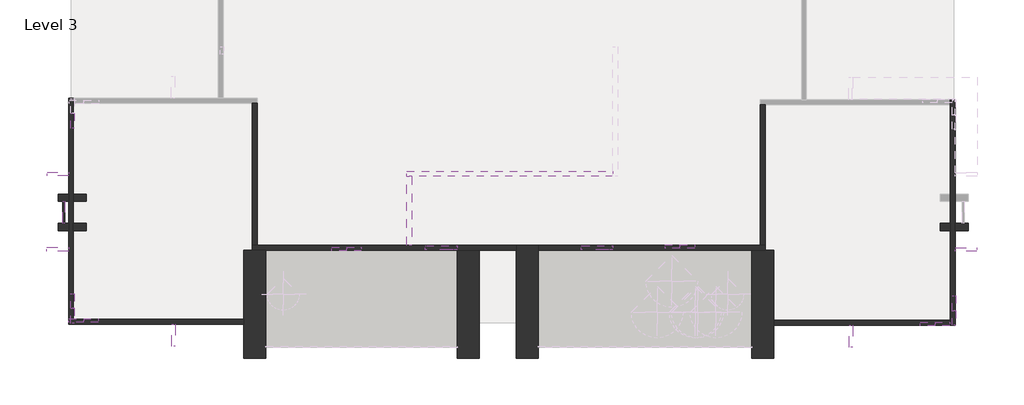
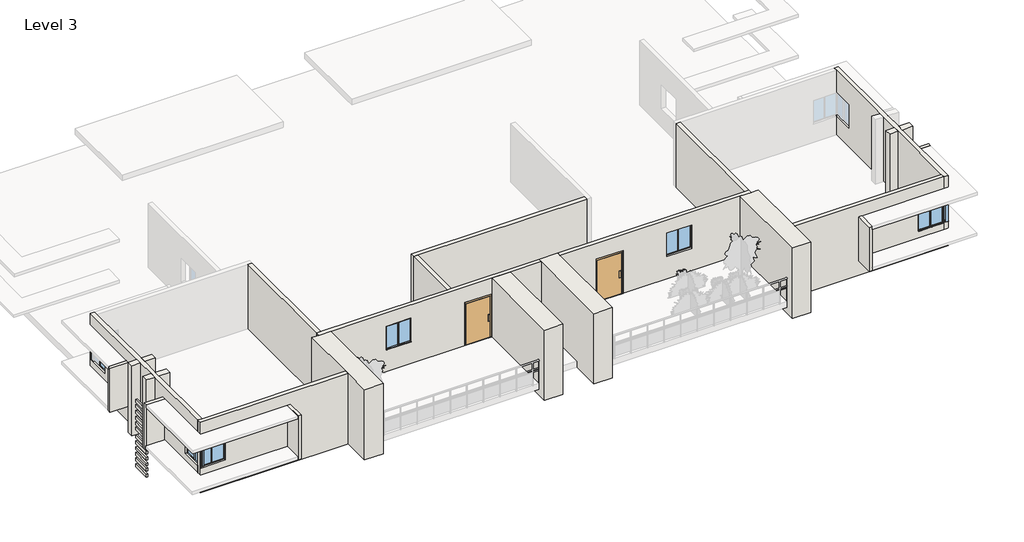
# One storey, part 1 of 4: 49 walls, 13 windows, 2 doors.
"""IFC4 building model written with IfcOpenShell, lengths in millimetres."""

from ifc_helpers import new_model, si_unit, frame, origin, place, context, project, spatial, polyline, outline, extrude, faceted_brep, transform, mapped, element, save
from components import door_15d3c954, window_20ff4747

model = new_model("IFC4")

# Units and contexts
model_context = context("Model", 3, world=origin())
ifc_project = project(units=[si_unit("LENGTHUNIT", "METRE", prefix="MILLI")], contexts=[model_context])

# Site, building, storey
site = spatial("IfcSite", under=ifc_project)
building = spatial("IfcBuilding", under=site)
storey = spatial("IfcBuildingStorey", under=building, Name="Level 3", Elevation=6096.0)

# Doors
placement = place(None, origin())
door_shape = door_15d3c954(model_context)
element("IfcDoor", 1, ObjectType="Door-Passage-Single-Flush-Dbl_Acting : 48\" x 96\"", at=placement, inside=storey, context=model_context, shape_type="MappedRepresentation", body=[
    mapped(door_shape, transform((7011.0520665, -5255.880811, 7315.2), x_axis=(-1.0, 0.0, 0.0), y_axis=(0.0, -1.0, 0.0), z_axis=(0.0, 0.0, 1.0))),
])
element("IfcDoor", 2, ObjectType="Door-Passage-Single-Flush-Dbl_Acting : 48\" x 96\"", at=placement, inside=storey, context=model_context, shape_type="MappedRepresentation", body=[
    mapped(door_shape, transform((559.4520665, -5255.1961695, 7315.2), x_axis=(-1.0, 0.0, 0.0), y_axis=(0.0, -1.0, 0.0), z_axis=(0.0, 0.0, 1.0))),
])

# Walls
element("IfcWall", 3, ObjectType="Generic - 1'", at=placement, inside=storey, context=model_context, shape_type="SweptSolid", body=[
    extrude(outline(polyline([(-14151.7972154, -3343.5294056), (-14680.5479335, -3343.5294056), (-14680.5479335, -3038.7294056), (-14151.7972154, -3038.7294056), (-14151.7972154, -3343.5294056)])), frame((0.0, 0.0, 6705.6), z_axis=(0.0, 0.0, 1.0), x_axis=(1.0, 0.0, 0.0)), (0.0, 0.0, 1.0), 3657.6),
])
element("IfcWall", 4, ObjectType="Generic - 1'", at=placement, inside=storey, context=model_context, shape_type="SweptSolid", body=[
    extrude(outline(polyline([(-15302.1394029, -3038.7294056), (-14883.7479335, -3038.7294056), (-14883.7479335, -3343.5294056), (-15302.1394029, -3343.5294056), (-15302.1394029, -3038.7294056)])), frame((0.0, 0.0, 6705.6), z_axis=(0.0, 0.0, 1.0), x_axis=(1.0, 0.0, 0.0)), (0.0, 0.0, 1.0), 3657.6),
])
element("IfcWall", 5, ObjectType="Generic - 1'", at=placement, inside=storey, context=model_context, shape_type="SweptSolid", body=[
    extrude(outline(polyline([(-14151.7972154, -4562.7294056), (-14680.5479335, -4562.7294056), (-14680.5479335, -4257.9294056), (-14151.7972154, -4257.9294056), (-14151.7972154, -4562.7294056)])), frame((0.0, 0.0, 6705.6), z_axis=(0.0, 0.0, 1.0), x_axis=(1.0, 0.0, 0.0)), (0.0, 0.0, 1.0), 3657.6),
])
element("IfcWall", 6, ObjectType="Generic - 1'", at=placement, inside=storey, context=model_context, shape_type="SweptSolid", body=[
    extrude(outline(polyline([(-15302.1394029, -4257.9294056), (-14883.7479335, -4257.9294056), (-14883.7479335, -4562.7294056), (-15302.1394029, -4562.7294056), (-15302.1394029, -4257.9294056)])), frame((0.0, 0.0, 6705.6), z_axis=(0.0, 0.0, 1.0), x_axis=(1.0, 0.0, 0.0)), (0.0, 0.0, 1.0), 3657.6),
])
element("IfcWall", 7, ObjectType="Generic - 1'", at=placement, inside=storey, context=model_context, shape_type="SweptSolid", body=[
    extrude(outline(polyline([(22386.1027846, -4562.7294056), (21857.3520665, -4562.7294056), (21857.3520665, -4257.9294056), (22386.1027846, -4257.9294056), (22386.1027846, -4562.7294056)])), frame((0.0, 0.0, 6705.6), z_axis=(0.0, 0.0, 1.0), x_axis=(1.0, 0.0, 0.0)), (0.0, 0.0, 1.0), 3657.6),
])
element("IfcWall", 8, ObjectType="Generic - 1'", at=placement, inside=storey, context=model_context, shape_type="SweptSolid", body=[
    extrude(outline(polyline([(21235.7605971, -4257.9294056), (21654.1520665, -4257.9294056), (21654.1520665, -4562.7294056), (21235.7605971, -4562.7294056), (21235.7605971, -4257.9294056)])), frame((0.0, 0.0, 6705.6), z_axis=(0.0, 0.0, 1.0), x_axis=(1.0, 0.0, 0.0)), (0.0, 0.0, 1.0), 3657.6),
])
element("IfcWall", 9, ObjectType="Generic - 3'", at=placement, inside=storey, context=model_context, shape_type="Brep", body=[
    faceted_brep([(2134.2520665, -9833.5461695, 6705.6), (2134.2520665, -5363.1461695, 6705.6), (2134.2520665, -5363.1461695, 10363.2), (2134.2520665, -9833.5461695, 10363.2), (1219.8520665, -9833.5461695, 6705.6), (1219.8520665, -9833.5461695, 10363.2), (1219.8520665, -5363.1461695, 10363.2), (1219.8520665, -5363.1461695, 9550.4), (1219.8520665, -5363.1461695, 7315.2), (1219.8520665, -5363.1461695, 6705.6)], [[[0, 1, 2, 3]], [[4, 5, 6, 7, 8, 9]], [[1, 0, 4, 9]], [[3, 2, 6, 5]], [[0, 3, 5, 4]], [[2, 1, 9, 8, 7, 6]]]),
])
element("IfcWall", 10, ObjectType="Generic - 3'", at=placement, inside=storey, context=model_context, shape_type="Brep", body=[
    faceted_brep([(4572.6520665, -9833.5461695, 6705.6), (4572.6520665, -5363.830811, 6705.6), (4572.6520665, -5160.630811, 6705.6), (4572.6520665, -5160.630811, 10363.2), (4572.6520665, -5363.830811, 10363.2), (4572.6520665, -9833.5461695, 10363.2), (3658.2520665, -9833.5461695, 6705.6), (3658.2520665, -9833.5461695, 10363.2), (3658.2520665, -5363.1461695, 10363.2), (3658.2520665, -5160.630811, 10363.2), (3658.2520665, -5160.630811, 6705.6), (3658.2520665, -5363.1461695, 6705.6)], [[[0, 1, 2, 3, 4, 5]], [[6, 7, 8, 9, 10, 11]], [[2, 1, 0, 6, 11, 10]], [[5, 4, 3, 9, 8, 7]], [[0, 5, 7, 6]], [[3, 2, 10, 9]]]),
])
element("IfcWall", 11, ObjectType="Generic - 3'", at=placement, inside=storey, context=model_context, shape_type="Brep", body=[
    faceted_brep([(-7619.3479335, -5363.1461695, 6705.6), (-7619.3479335, -8237.0604699, 6705.6), (-7619.3479335, -8440.2604699, 6705.6), (-7619.3479335, -9833.5461695, 6705.6), (-7619.3479335, -9833.5461695, 10363.2), (-7619.3479335, -8440.2604699, 10363.2), (-7619.3479335, -8237.0604699, 10363.2), (-7619.3479335, -5363.1461695, 10363.2), (-6704.9479335, -5363.1461695, 6705.6), (-6704.9479335, -5363.1461695, 10363.2), (-6704.9479335, -9833.5461695, 10363.2), (-6704.9479335, -9833.5461695, 6705.6), (-7263.7479335, -5363.1461695, 6705.6), (-7263.7479335, -5363.1461695, 10363.2)], [[[0, 1, 2, 3, 4, 5, 6, 7]], [[8, 9, 10, 11]], [[3, 2, 1, 0, 12, 8, 11]], [[4, 3, 11, 10]], [[7, 6, 5, 4, 10, 9, 13]], [[0, 7, 13, 9, 8, 12]]]),
])
element("IfcWall", 12, ObjectType="Generic - 3'", at=placement, inside=storey, context=model_context, shape_type="Brep", body=[
    faceted_brep([(13411.8520665, -5363.830811, 6705.6), (13411.8520665, -9834.230811, 6705.6), (13411.8520665, -9834.230811, 10363.2), (13411.8520665, -5363.830811, 10363.2), (14326.2520665, -5363.830811, 6705.6), (14326.2520665, -5363.830811, 10363.2), (14326.2520665, -8263.1451114, 10363.2), (14326.2520665, -8466.3451114, 10363.2), (14326.2520665, -9834.230811, 10363.2), (14326.2520665, -9834.230811, 6705.6), (14326.2520665, -8466.3451114, 6705.6), (14326.2520665, -8263.1451114, 6705.6), (13970.6520665, -5363.830811, 6705.6), (13970.6520665, -5363.830811, 10363.2)], [[[0, 1, 2, 3]], [[4, 5, 6, 7, 8, 9, 10, 11]], [[1, 0, 12, 4, 11, 10, 9]], [[2, 1, 9, 8]], [[3, 2, 8, 7, 6, 5, 13]], [[0, 3, 13, 5, 4, 12]]]),
])
element("IfcWall", 13, ObjectType="Generic - 5\"", at=placement, inside=storey, context=model_context, shape_type="SweptSolid", body=[
    extrude(outline(polyline([(-15124.6936682, -4257.9294056), (-15124.6936682, -3343.5294056), (-15048.4936682, -3343.5294056), (-15048.4936682, -4257.9294056), (-15124.6936682, -4257.9294056)])), frame((0.0, 0.0, 5054.6), z_axis=(0.0, 0.0, 1.0), x_axis=(1.0, 0.0, 0.0)), (0.0, 0.0, 1.0), 152.8735856),
])
element("IfcWall", 14, ObjectType="Generic - 5\"", at=placement, inside=storey, context=model_context, shape_type="SweptSolid", body=[
    extrude(outline(polyline([(-15124.6936682, -4257.9294056), (-15124.6936682, -3343.5294056), (-15048.4936682, -3343.5294056), (-15048.4936682, -4257.9294056), (-15124.6936682, -4257.9294056)])), frame((0.0, 0.0, 5359.4), z_axis=(0.0, 0.0, 1.0), x_axis=(1.0, 0.0, 0.0)), (0.0, 0.0, 1.0), 152.8735856),
])
element("IfcWall", 15, ObjectType="Generic - 5\"", at=placement, inside=storey, context=model_context, shape_type="SweptSolid", body=[
    extrude(outline(polyline([(-15124.6936682, -4257.9294056), (-15124.6936682, -3343.5294056), (-15048.4936682, -3343.5294056), (-15048.4936682, -4257.9294056), (-15124.6936682, -4257.9294056)])), frame((0.0, 0.0, 5638.8), z_axis=(0.0, 0.0, 1.0), x_axis=(1.0, 0.0, 0.0)), (0.0, 0.0, 1.0), 152.8735856),
])
element("IfcWall", 16, ObjectType="Generic - 5\"", at=placement, inside=storey, context=model_context, shape_type="SweptSolid", body=[
    extrude(outline(polyline([(-15124.6936682, -4257.9294056), (-15124.6936682, -3343.5294056), (-15048.4936682, -3343.5294056), (-15048.4936682, -4257.9294056), (-15124.6936682, -4257.9294056)])), frame((0.0, 0.0, 5943.6), z_axis=(0.0, 0.0, 1.0), x_axis=(1.0, 0.0, 0.0)), (0.0, 0.0, 1.0), 152.8735856),
])
element("IfcWall", 17, ObjectType="Generic - 5\"", at=placement, inside=storey, context=model_context, shape_type="SweptSolid", body=[
    extrude(outline(polyline([(-15124.6936682, -4257.9294056), (-15124.6936682, -3343.5294056), (-15048.4936682, -3343.5294056), (-15048.4936682, -4257.9294056), (-15124.6936682, -4257.9294056)])), frame((0.0, 0.0, 6248.4), z_axis=(0.0, 0.0, 1.0), x_axis=(1.0, 0.0, 0.0)), (0.0, 0.0, 1.0), 152.8735856),
])
element("IfcWall", 18, ObjectType="Generic - 5\"", at=placement, inside=storey, context=model_context, shape_type="SweptSolid", body=[
    extrude(outline(polyline([(-15124.6936682, -4257.9294056), (-15124.6936682, -3343.5294056), (-15048.4936682, -3343.5294056), (-15048.4936682, -4257.9294056), (-15124.6936682, -4257.9294056)])), frame((0.0, 0.0, 6553.2), z_axis=(0.0, 0.0, 1.0), x_axis=(1.0, 0.0, 0.0)), (0.0, 0.0, 1.0), 152.8735856),
])
element("IfcWall", 19, ObjectType="Generic - 5\"", at=placement, inside=storey, context=model_context, shape_type="SweptSolid", body=[
    extrude(outline(polyline([(-15124.6936682, -4257.9294056), (-15124.6936682, -3343.5294056), (-15048.4936682, -3343.5294056), (-15048.4936682, -4257.9294056), (-15124.6936682, -4257.9294056)])), frame((0.0, 0.0, 5054.6), z_axis=(0.0, 0.0, 1.0), x_axis=(1.0, 0.0, 0.0)), (0.0, 0.0, 1.0), 152.8735856),
])
element("IfcWall", 20, ObjectType="Generic - 5\"", at=placement, inside=storey, context=model_context, shape_type="SweptSolid", body=[
    extrude(outline(polyline([(-15124.6936682, -4257.9294056), (-15124.6936682, -3343.5294056), (-15048.4936682, -3343.5294056), (-15048.4936682, -4257.9294056), (-15124.6936682, -4257.9294056)])), frame((0.0, 0.0, 5359.4), z_axis=(0.0, 0.0, 1.0), x_axis=(1.0, 0.0, 0.0)), (0.0, 0.0, 1.0), 152.8735856),
])
element("IfcWall", 21, ObjectType="Generic - 5\"", at=placement, inside=storey, context=model_context, shape_type="SweptSolid", body=[
    extrude(outline(polyline([(-15124.6936682, -4257.9294056), (-15124.6936682, -3343.5294056), (-15048.4936682, -3343.5294056), (-15048.4936682, -4257.9294056), (-15124.6936682, -4257.9294056)])), frame((0.0, 0.0, 5638.8), z_axis=(0.0, 0.0, 1.0), x_axis=(1.0, 0.0, 0.0)), (0.0, 0.0, 1.0), 152.8735856),
])
element("IfcWall", 22, ObjectType="Generic - 5\"", at=placement, inside=storey, context=model_context, shape_type="SweptSolid", body=[
    extrude(outline(polyline([(-15124.6936682, -4257.9294056), (-15124.6936682, -3343.5294056), (-15048.4936682, -3343.5294056), (-15048.4936682, -4257.9294056), (-15124.6936682, -4257.9294056)])), frame((0.0, 0.0, 5943.6), z_axis=(0.0, 0.0, 1.0), x_axis=(1.0, 0.0, 0.0)), (0.0, 0.0, 1.0), 152.8735856),
])
element("IfcWall", 23, ObjectType="Generic - 5\"", at=placement, inside=storey, context=model_context, shape_type="SweptSolid", body=[
    extrude(outline(polyline([(-15124.6936682, -4257.9294056), (-15124.6936682, -3343.5294056), (-15048.4936682, -3343.5294056), (-15048.4936682, -4257.9294056), (-15124.6936682, -4257.9294056)])), frame((0.0, 0.0, 6248.4), z_axis=(0.0, 0.0, 1.0), x_axis=(1.0, 0.0, 0.0)), (0.0, 0.0, 1.0), 152.8735856),
])
element("IfcWall", 24, ObjectType="Generic - 5\"", at=placement, inside=storey, context=model_context, shape_type="SweptSolid", body=[
    extrude(outline(polyline([(-15124.6936682, -4257.9294056), (-15124.6936682, -3343.5294056), (-15048.4936682, -3343.5294056), (-15048.4936682, -4257.9294056), (-15124.6936682, -4257.9294056)])), frame((0.0, 0.0, 6553.2), z_axis=(0.0, 0.0, 1.0), x_axis=(1.0, 0.0, 0.0)), (0.0, 0.0, 1.0), 152.8735856),
])
element("IfcWall", 25, ObjectType="Generic - 5\"", at=placement, inside=storey, context=model_context, shape_type="SweptSolid", body=[
    extrude(outline(polyline([(-15124.6936682, -4257.9294056), (-15124.6936682, -3343.5294056), (-15048.4936682, -3343.5294056), (-15048.4936682, -4257.9294056), (-15124.6936682, -4257.9294056)])), frame((0.0, 0.0, 6959.6), z_axis=(0.0, 0.0, 1.0), x_axis=(1.0, 0.0, 0.0)), (0.0, 0.0, 1.0), 152.8735856),
])
element("IfcWall", 26, ObjectType="Generic - 5\"", at=placement, inside=storey, context=model_context, shape_type="SweptSolid", body=[
    extrude(outline(polyline([(-15124.6936682, -4257.9294056), (-15124.6936682, -3343.5294056), (-15048.4936682, -3343.5294056), (-15048.4936682, -4257.9294056), (-15124.6936682, -4257.9294056)])), frame((0.0, 0.0, 7239.0), z_axis=(0.0, 0.0, 1.0), x_axis=(1.0, 0.0, 0.0)), (0.0, 0.0, 1.0), 152.8735856),
])
element("IfcWall", 27, ObjectType="Generic - 5\"", at=placement, inside=storey, context=model_context, shape_type="SweptSolid", body=[
    extrude(outline(polyline([(-15124.6936682, -4257.9294056), (-15124.6936682, -3343.5294056), (-15048.4936682, -3343.5294056), (-15048.4936682, -4257.9294056), (-15124.6936682, -4257.9294056)])), frame((0.0, 0.0, 7518.4), z_axis=(0.0, 0.0, 1.0), x_axis=(1.0, 0.0, 0.0)), (0.0, 0.0, 1.0), 152.8735856),
])
element("IfcWall", 28, ObjectType="Generic - 5\"", at=placement, inside=storey, context=model_context, shape_type="SweptSolid", body=[
    extrude(outline(polyline([(-15124.6936682, -4257.9294056), (-15124.6936682, -3343.5294056), (-15048.4936682, -3343.5294056), (-15048.4936682, -4257.9294056), (-15124.6936682, -4257.9294056)])), frame((0.0, 0.0, 7823.2), z_axis=(0.0, 0.0, 1.0), x_axis=(1.0, 0.0, 0.0)), (0.0, 0.0, 1.0), 152.8735856),
])
element("IfcWall", 29, ObjectType="Generic - 5\"", at=placement, inside=storey, context=model_context, shape_type="SweptSolid", body=[
    extrude(outline(polyline([(-15124.6936682, -4257.9294056), (-15124.6936682, -3343.5294056), (-15048.4936682, -3343.5294056), (-15048.4936682, -4257.9294056), (-15124.6936682, -4257.9294056)])), frame((0.0, 0.0, 8128.0), z_axis=(0.0, 0.0, 1.0), x_axis=(1.0, 0.0, 0.0)), (0.0, 0.0, 1.0), 152.8735856),
])
element("IfcWall", 30, ObjectType="Generic - 5\"", at=placement, inside=storey, context=model_context, shape_type="SweptSolid", body=[
    extrude(outline(polyline([(-15124.6936682, -4257.9294056), (-15124.6936682, -3343.5294056), (-15048.4936682, -3343.5294056), (-15048.4936682, -4257.9294056), (-15124.6936682, -4257.9294056)])), frame((0.0, 0.0, 8407.4), z_axis=(0.0, 0.0, 1.0), x_axis=(1.0, 0.0, 0.0)), (0.0, 0.0, 1.0), 152.8735856),
])
element("IfcWall", 31, ObjectType="Generic - 5\"", at=placement, inside=storey, context=model_context, shape_type="SweptSolid", body=[
    extrude(outline(polyline([(-15124.6936682, -4257.9294056), (-15124.6936682, -3343.5294056), (-15048.4936682, -3343.5294056), (-15048.4936682, -4257.9294056), (-15124.6936682, -4257.9294056)])), frame((0.0, 0.0, 6959.6), z_axis=(0.0, 0.0, 1.0), x_axis=(1.0, 0.0, 0.0)), (0.0, 0.0, 1.0), 152.8735856),
])
element("IfcWall", 32, ObjectType="Generic - 5\"", at=placement, inside=storey, context=model_context, shape_type="SweptSolid", body=[
    extrude(outline(polyline([(-15124.6936682, -4257.9294056), (-15124.6936682, -3343.5294056), (-15048.4936682, -3343.5294056), (-15048.4936682, -4257.9294056), (-15124.6936682, -4257.9294056)])), frame((0.0, 0.0, 7239.0), z_axis=(0.0, 0.0, 1.0), x_axis=(1.0, 0.0, 0.0)), (0.0, 0.0, 1.0), 152.8735856),
])
element("IfcWall", 33, ObjectType="Generic - 5\"", at=placement, inside=storey, context=model_context, shape_type="SweptSolid", body=[
    extrude(outline(polyline([(-15124.6936682, -4257.9294056), (-15124.6936682, -3343.5294056), (-15048.4936682, -3343.5294056), (-15048.4936682, -4257.9294056), (-15124.6936682, -4257.9294056)])), frame((0.0, 0.0, 7518.4), z_axis=(0.0, 0.0, 1.0), x_axis=(1.0, 0.0, 0.0)), (0.0, 0.0, 1.0), 152.8735856),
])
element("IfcWall", 34, ObjectType="Generic - 5\"", at=placement, inside=storey, context=model_context, shape_type="SweptSolid", body=[
    extrude(outline(polyline([(-15124.6936682, -4257.9294056), (-15124.6936682, -3343.5294056), (-15048.4936682, -3343.5294056), (-15048.4936682, -4257.9294056), (-15124.6936682, -4257.9294056)])), frame((0.0, 0.0, 7823.2), z_axis=(0.0, 0.0, 1.0), x_axis=(1.0, 0.0, 0.0)), (0.0, 0.0, 1.0), 152.8735856),
])
element("IfcWall", 35, ObjectType="Generic - 5\"", at=placement, inside=storey, context=model_context, shape_type="SweptSolid", body=[
    extrude(outline(polyline([(-15124.6936682, -4257.9294056), (-15124.6936682, -3343.5294056), (-15048.4936682, -3343.5294056), (-15048.4936682, -4257.9294056), (-15124.6936682, -4257.9294056)])), frame((0.0, 0.0, 8128.0), z_axis=(0.0, 0.0, 1.0), x_axis=(1.0, 0.0, 0.0)), (0.0, 0.0, 1.0), 152.8735856),
])
element("IfcWall", 36, ObjectType="Generic - 5\"", at=placement, inside=storey, context=model_context, shape_type="SweptSolid", body=[
    extrude(outline(polyline([(-15124.6936682, -4257.9294056), (-15124.6936682, -3343.5294056), (-15048.4936682, -3343.5294056), (-15048.4936682, -4257.9294056), (-15124.6936682, -4257.9294056)])), frame((0.0, 0.0, 8407.4), z_axis=(0.0, 0.0, 1.0), x_axis=(1.0, 0.0, 0.0)), (0.0, 0.0, 1.0), 152.8735856),
])
element("IfcWall", 37, ObjectType="Generic - 6\"", at=placement, inside=storey, context=model_context, shape_type="SweptSolid", body=[
    extrude(outline(polyline([(22749.4138484, -5418.3451114), (21857.3520665, -5418.3451114), (21857.3520665, -5265.9451114), (22749.4138484, -5265.9451114), (22749.4138484, -5418.3451114)])), frame((0.0, 0.0, 7467.6), z_axis=(0.0, 0.0, 1.0), x_axis=(1.0, 0.0, 0.0)), (0.0, 0.0, 1.0), 2286.0),
])
element("IfcWall", 38, ObjectType="Generic - 6\"", at=placement, inside=storey, context=model_context, shape_type="SweptSolid", body=[
    extrude(outline(polyline([(17454.3075984, -9380.7451114), (17454.3075984, -8466.3451114), (17606.7075984, -8466.3451114), (17606.7075984, -9380.7451114), (17454.3075984, -9380.7451114)])), frame((0.0, 0.0, 7467.6), z_axis=(0.0, 0.0, 1.0), x_axis=(1.0, 0.0, 0.0)), (0.0, 0.0, 1.0), 2286.0),
])
element("IfcWall", 39, ObjectType="Generic - 6\"", at=placement, inside=storey, context=model_context, shape_type="SweptSolid", body=[
    extrude(outline(polyline([(-15775.8097154, -2128.3604699), (-14883.7479335, -2128.3604699), (-14883.7479335, -2280.7604699), (-15775.8097154, -2280.7604699), (-15775.8097154, -2128.3604699)])), frame((0.0, 0.0, 7467.6), z_axis=(0.0, 0.0, 1.0), x_axis=(1.0, 0.0, 0.0)), (0.0, 0.0, 1.0), 2286.0),
])
element("IfcWall", 40, ObjectType="Generic - 6\"", at=placement, inside=storey, context=model_context, shape_type="SweptSolid", body=[
    extrude(outline(polyline([(-15796.5604335, -5250.9729699), (-14883.7479335, -5250.9729699), (-14883.7479335, -5403.3729699), (-15796.5604335, -5403.3729699), (-15796.5604335, -5250.9729699)])), frame((0.0, 0.0, 7467.6), z_axis=(0.0, 0.0, 1.0), x_axis=(1.0, 0.0, 0.0)), (0.0, 0.0, 1.0), 2286.0),
])
element("IfcWall", 41, ObjectType="Generic - 6\"", at=placement, inside=storey, context=model_context, shape_type="SweptSolid", body=[
    extrude(outline(polyline([(-10607.7034654, -9354.6604699), (-10607.7034654, -8440.2604699), (-10455.3034654, -8440.2604699), (-10455.3034654, -9354.6604699), (-10607.7034654, -9354.6604699)])), frame((0.0, 0.0, 7467.6), z_axis=(0.0, 0.0, 1.0), x_axis=(1.0, 0.0, 0.0)), (0.0, 0.0, 1.0), 2286.0),
])
element("IfcWall", 42, ObjectType="Generic - 8\"", at=placement, inside=storey, context=model_context, shape_type="Brep", body=[
    faceted_brep([(7671.4520665, -2102.9604699, 7315.2), (-862.9479335, -2102.9604699, 7315.2), (-862.9479335, -2102.9604699, 10363.2), (7671.4520665, -2102.9604699, 10363.2), (7671.4520665, -2306.1604699, 7315.2), (7671.4520665, -2306.1604699, 10363.2), (-659.7479335, -2306.1604699, 10363.2), (-862.9479335, -2306.1604699, 10363.2), (-862.9479335, -2306.1604699, 7315.2), (-659.7479335, -2306.1604699, 7315.2)], [[[0, 1, 2, 3]], [[4, 5, 6, 7, 8, 9]], [[1, 0, 4, 9, 8]], [[3, 2, 7, 6, 5]], [[0, 3, 5, 4]], [[2, 1, 8, 7]]]),
])
element("IfcWall", 43, ObjectType="Generic - 8\"", at=placement, inside=storey, context=model_context, shape_type="SweptSolid", body=[
    extrude(outline(polyline([(-862.9479335, -5159.9461695), (-862.9479335, -2306.1604699), (-659.7479335, -2306.1604699), (-659.7479335, -5159.9461695), (-862.9479335, -5159.9461695)])), frame((0.0, 0.0, 7315.2), z_axis=(0.0, 0.0, 1.0), x_axis=(1.0, 0.0, 0.0)), (0.0, 0.0, 1.0), 3048.0),
])
element("IfcWall", 44, ObjectType="Generic - 8\" gray", at=placement, inside=storey, context=model_context, shape_type="Brep", body=[
    faceted_brep([(-14883.7479335, -8440.2604699, 6705.6), (-7619.3479335, -8440.2604699, 6705.6), (-7619.3479335, -8440.2604699, 10363.2), (-14883.7479335, -8440.2604699, 10363.2), (-13655.3509584, -8440.2604699, 7977.8804451), (-14874.5509584, -8440.2604699, 7977.8804451), (-14874.5509584, -8440.2604699, 9197.0804451), (-13655.3509584, -8440.2604699, 9197.0804451), (-7619.3479335, -8237.0604699, 6705.6), (-14680.5479335, -8237.0604699, 6705.6), (-14883.7479335, -8237.0604699, 6705.6), (-14883.7479335, -8237.0604699, 7977.8804451), (-14883.7479335, -8237.0604699, 9197.0804451), (-14883.7479335, -8237.0604699, 10363.2), (-14680.5479335, -8237.0604699, 10363.2), (-7619.3479335, -8237.0604699, 10363.2), (-14874.5509584, -8237.0604699, 7977.8804451), (-14680.5479335, -8237.0604699, 7977.8804451), (-13655.3509584, -8237.0604699, 7977.8804451), (-13655.3509584, -8237.0604699, 9197.0804451), (-14680.5479335, -8237.0604699, 9197.0804451), (-14874.5509584, -8237.0604699, 9197.0804451)], [[[0, 1, 2, 3], [4, 5, 6, 7]], [[8, 9, 10, 11, 12, 13, 14, 15], [16, 17, 18, 19, 20, 21]], [[1, 0, 10, 9, 8]], [[3, 2, 15, 14, 13]], [[0, 3, 13, 12, 11, 10]], [[2, 1, 8, 15]], [[4, 18, 17, 16, 5]], [[6, 5, 16, 21]], [[6, 21, 20, 19, 7]], [[7, 19, 18, 4]]]),
])
element("IfcWall", 45, ObjectType="Generic - 8\" gray", at=placement, inside=storey, context=model_context, shape_type="Brep", body=[
    faceted_brep([(-14883.7479335, 919.6395301, 6705.6), (-14883.7479335, -3038.7294056, 6705.6), (-14883.7479335, -3343.5294056, 6705.6), (-14883.7479335, -4257.9294056, 6705.6), (-14883.7479335, -4562.7294056, 6705.6), (-14883.7479335, -8237.0604699, 6705.6), (-14883.7479335, -8237.0604699, 7977.8804451), (-14883.7479335, -7169.263768, 7977.8804451), (-14883.7479335, -7169.263768, 9197.0804451), (-14883.7479335, -8237.0604699, 9197.0804451), (-14883.7479335, -8237.0604699, 10363.2), (-14883.7479335, -4562.7294056, 10363.2), (-14883.7479335, -4257.9294056, 10363.2), (-14883.7479335, -3343.5294056, 10363.2), (-14883.7479335, -3038.7294056, 10363.2), (-14883.7479335, 919.6395301, 10363.2), (-14883.7479335, -310.2864811, 7977.8804451), (-14883.7479335, 908.9135189, 7977.8804451), (-14883.7479335, 908.9135189, 9197.0804451), (-14883.7479335, -310.2864811, 9197.0804451), (-14680.5479335, -8237.0604699, 6705.6), (-14680.5479335, -4562.7294056, 6705.6), (-14680.5479335, -4257.9294056, 6705.6), (-14680.5479335, -3343.5294056, 6705.6), (-14680.5479335, -3038.7294056, 6705.6), (-14680.5479335, 716.4395301, 6705.6), (-14680.5479335, 919.6395301, 6705.6), (-14680.5479335, 919.6395301, 7977.8804451), (-14680.5479335, 919.6395301, 9197.0804451), (-14680.5479335, 919.6395301, 10363.2), (-14680.5479335, 716.4395301, 10363.2), (-14680.5479335, -3038.7294056, 10363.2), (-14680.5479335, -3343.5294056, 10363.2), (-14680.5479335, -4257.9294056, 10363.2), (-14680.5479335, -4562.7294056, 10363.2), (-14680.5479335, -8237.0604699, 10363.2), (-14680.5479335, -8237.0604699, 9197.0804451), (-14680.5479335, -7169.263768, 9197.0804451), (-14680.5479335, -7169.263768, 7977.8804451), (-14680.5479335, -8237.0604699, 7977.8804451), (-14680.5479335, 908.9135189, 7977.8804451), (-14680.5479335, 716.4395301, 7977.8804451), (-14680.5479335, -310.2864811, 7977.8804451), (-14680.5479335, -310.2864811, 9197.0804451), (-14680.5479335, 716.4395301, 9197.0804451), (-14680.5479335, 908.9135189, 9197.0804451), (-14874.5509584, -8237.0604699, 7977.8804451), (-14874.5509584, -8237.0604699, 9197.0804451)], [[[0, 1, 2, 3, 4, 5, 6, 7, 8, 9, 10, 11, 12, 13, 14, 15], [16, 17, 18, 19]], [[20, 21, 22, 23, 24, 25, 26, 27, 28, 29, 30, 31, 32, 33, 34, 35, 36, 37, 38, 39], [40, 41, 42, 43, 44, 45]], [[5, 4, 3, 2, 1, 0, 26, 25, 24, 23, 22, 21, 20]], [[15, 14, 13, 12, 11, 10, 35, 34, 33, 32, 31, 30, 29]], [[0, 15, 29, 28, 27, 26]], [[5, 20, 39, 46, 6]], [[35, 10, 9, 47, 36]], [[38, 7, 6, 46, 39]], [[8, 7, 38, 37]], [[8, 37, 36, 47, 9]], [[16, 42, 41, 40, 17]], [[18, 45, 44, 43, 19]], [[19, 43, 42, 16]], [[45, 18, 17, 40]]]),
])
element("IfcWall", 46, ObjectType="Generic - 8\" gray", at=placement, inside=storey, context=model_context, shape_type="Brep", body=[
    faceted_brep([(21654.1520665, 868.1548886, 6705.6), (21654.1520665, 664.9548886, 6705.6), (21654.1520665, -3038.7294056, 6705.6), (21654.1520665, -3343.5294056, 6705.6), (21654.1520665, -4257.9294056, 6705.6), (21654.1520665, -4562.7294056, 6705.6), (21654.1520665, -8263.1451114, 6705.6), (21654.1520665, -8466.3451114, 6705.6), (21654.1520665, -8466.3451114, 7977.8804451), (21654.1520665, -7262.9130582, 7977.8804451), (21654.1520665, -7262.9130582, 9197.0804451), (21654.1520665, -8466.3451114, 9197.0804451), (21654.1520665, -8466.3451114, 10363.2), (21654.1520665, -8263.1451114, 10363.2), (21654.1520665, -4562.7294056, 10363.2), (21654.1520665, -4257.9294056, 10363.2), (21654.1520665, -3343.5294056, 10363.2), (21654.1520665, -3038.7294056, 10363.2), (21654.1520665, 664.9548886, 10363.2), (21654.1520665, 868.1548886, 10363.2), (21654.1520665, 868.1548886, 9197.0804451), (21654.1520665, 868.1548886, 7977.8804451), (21654.1520665, 859.364485, 7977.8804451), (21654.1520665, 859.364485, 9197.0804451), (21654.1520665, 664.9548886, 9197.0804451), (21654.1520665, -359.835515, 9197.0804451), (21654.1520665, -359.835515, 7977.8804451), (21654.1520665, 664.9548886, 7977.8804451), (21857.3520665, -8466.3451114, 6705.6), (21857.3520665, -4562.7294056, 6705.6), (21857.3520665, -4257.9294056, 6705.6), (21857.3520665, -3343.5294056, 6705.6), (21857.3520665, -3038.7294056, 6705.6), (21857.3520665, 868.1548886, 6705.6), (21857.3520665, 868.1548886, 10363.2), (21857.3520665, -3038.7294056, 10363.2), (21857.3520665, -3343.5294056, 10363.2), (21857.3520665, -4257.9294056, 10363.2), (21857.3520665, -4562.7294056, 10363.2), (21857.3520665, -8466.3451114, 10363.2), (21857.3520665, -8466.3451114, 9197.0804451), (21857.3520665, -7262.9130582, 9197.0804451), (21857.3520665, -7262.9130582, 7977.8804451), (21857.3520665, -8466.3451114, 7977.8804451), (21857.3520665, 859.364485, 9197.0804451), (21857.3520665, 859.364485, 7977.8804451), (21857.3520665, -359.835515, 7977.8804451), (21857.3520665, -359.835515, 9197.0804451)], [[[0, 1, 2, 3, 4, 5, 6, 7, 8, 9, 10, 11, 12, 13, 14, 15, 16, 17, 18, 19, 20, 21], [22, 23, 24, 25, 26, 27]], [[28, 29, 30, 31, 32, 33, 34, 35, 36, 37, 38, 39, 40, 41, 42, 43], [44, 45, 46, 47]], [[7, 6, 5, 4, 3, 2, 1, 0, 33, 32, 31, 30, 29, 28]], [[19, 18, 17, 16, 15, 14, 13, 12, 39, 38, 37, 36, 35, 34]], [[0, 21, 20, 19, 34, 33]], [[7, 28, 43, 8]], [[39, 12, 11, 40]], [[45, 22, 27, 26, 46]], [[23, 22, 45, 44]], [[23, 44, 47, 25, 24]], [[25, 47, 46, 26]], [[8, 43, 42, 9]], [[10, 9, 42, 41]], [[10, 41, 40, 11]]]),
])
element("IfcWall", 47, ObjectType="Generic - 8\" gray", at=placement, inside=storey, context=model_context, shape_type="Brep", body=[
    faceted_brep([(3658.2520665, -5159.9461695, 6705.6), (-7060.5479335, -5159.9461695, 6705.6), (-7263.7479335, -5159.9461695, 6705.6), (-7263.7479335, -5159.9461695, 10363.2), (-7060.5479335, -5159.9461695, 10363.2), (-862.9479335, -5159.9461695, 10363.2), (-659.7479335, -5159.9461695, 10363.2), (3658.2520665, -5159.9461695, 10363.2), (-2753.0651847, -5159.9461695, 8454.6951112), (-2753.0651847, -5159.9461695, 9673.8951112), (-3972.2651847, -5159.9461695, 9673.8951112), (-3972.2651847, -5159.9461695, 8454.6951112), (-100.9479335, -5159.9461695, 9550.4), (-100.9479335, -5159.9461695, 7315.2), (1219.8520665, -5159.9461695, 7315.2), (1219.8520665, -5159.9461695, 9550.4), (-7263.7479335, -5363.1461695, 6705.6), (-6704.9479335, -5363.1461695, 6705.6), (1219.8520665, -5363.1461695, 6705.6), (2134.2520665, -5363.1461695, 6705.6), (3658.2520665, -5363.1461695, 6705.6), (3658.2520665, -5363.1461695, 10363.2), (2134.2520665, -5363.1461695, 10363.2), (1219.8520665, -5363.1461695, 10363.2), (-6704.9479335, -5363.1461695, 10363.2), (-7263.7479335, -5363.1461695, 10363.2), (-2753.0651847, -5363.1461695, 9673.8951112), (-2753.0651847, -5363.1461695, 8454.6951112), (-3972.2651847, -5363.1461695, 8454.6951112), (-3972.2651847, -5363.1461695, 9673.8951112), (-100.9479335, -5363.1461695, 7315.2), (-100.9479335, -5363.1461695, 9550.4), (1219.8520665, -5363.1461695, 9550.4), (1219.8520665, -5363.1461695, 7315.2), (3658.2520665, -5160.630811, 6705.6), (3658.2520665, -5160.630811, 10363.2)], [[[0, 1, 2, 3, 4, 5, 6, 7], [8, 9, 10, 11], [12, 13, 14, 15]], [[16, 17, 18, 19, 20, 21, 22, 23, 24, 25], [26, 27, 28, 29], [30, 31, 32, 33]], [[2, 1, 0, 34, 20, 19, 18, 17, 16]], [[7, 6, 5, 4, 3, 25, 24, 23, 22, 21, 35]], [[0, 7, 35, 21, 20, 34]], [[3, 2, 16, 25]], [[27, 8, 11, 28]], [[9, 8, 27, 26]], [[9, 26, 29, 10]], [[10, 29, 28, 11]], [[30, 13, 12, 31]], [[31, 12, 15, 32]], [[32, 15, 14, 33]], [[13, 30, 33, 14]]]),
])
element("IfcWall", 48, ObjectType="Generic - 8\" gray", at=placement, inside=storey, context=model_context, shape_type="Brep", body=[
    faceted_brep([(4572.6520665, -5363.830811, 6705.6), (13411.8520665, -5363.830811, 6705.6), (13970.6520665, -5363.830811, 6705.6), (13970.6520665, -5363.830811, 10363.2), (13411.8520665, -5363.830811, 10363.2), (4572.6520665, -5363.830811, 10363.2), (9831.9980014, -5363.830811, 8473.4493508), (9831.9980014, -5363.830811, 9692.6493508), (11051.1980014, -5363.830811, 9692.6493508), (11051.1980014, -5363.830811, 8473.4493508), (6350.6520665, -5363.830811, 7315.2), (6350.6520665, -5363.830811, 9550.4), (7671.4520665, -5363.830811, 9550.4), (7671.4520665, -5363.830811, 7315.2), (13970.6520665, -5160.630811, 6705.6), (13767.4520665, -5160.630811, 6705.6), (4572.6520665, -5160.630811, 6705.6), (4572.6520665, -5160.630811, 10363.2), (13767.4520665, -5160.630811, 10363.2), (13970.6520665, -5160.630811, 10363.2), (9831.9980014, -5160.630811, 9692.6493508), (9831.9980014, -5160.630811, 8473.4493508), (11051.1980014, -5160.630811, 8473.4493508), (11051.1980014, -5160.630811, 9692.6493508), (6350.6520665, -5160.630811, 9550.4), (6350.6520665, -5160.630811, 7315.2), (7671.4520665, -5160.630811, 7315.2), (7671.4520665, -5160.630811, 9550.4)], [[[0, 1, 2, 3, 4, 5], [6, 7, 8, 9], [10, 11, 12, 13]], [[14, 15, 16, 17, 18, 19], [20, 21, 22, 23], [24, 25, 26, 27]], [[2, 1, 0, 16, 15, 14]], [[5, 4, 3, 19, 18, 17]], [[0, 5, 17, 16]], [[3, 2, 14, 19]], [[21, 6, 9, 22]], [[7, 6, 21, 20]], [[7, 20, 23, 8]], [[8, 23, 22, 9]], [[10, 25, 24, 11]], [[11, 24, 27, 12]], [[12, 27, 26, 13]], [[25, 10, 13, 26]]]),
])
element("IfcWall", 49, ObjectType="Generic - 8\" gray", at=placement, inside=storey, context=model_context, shape_type="Brep", body=[
    faceted_brep([(21654.1520665, -8263.1451114, 6705.6), (14326.2520665, -8263.1451114, 6705.6), (14326.2520665, -8263.1451114, 10363.2), (21654.1520665, -8263.1451114, 10363.2), (20403.2295783, -8263.1451114, 7977.8804451), (21622.4295783, -8263.1451114, 7977.8804451), (21622.4295783, -8263.1451114, 9197.0804451), (20403.2295783, -8263.1451114, 9197.0804451), (14326.2520665, -8466.3451114, 6705.6), (21654.1520665, -8466.3451114, 6705.6), (21654.1520665, -8466.3451114, 7977.8804451), (21654.1520665, -8466.3451114, 9197.0804451), (21654.1520665, -8466.3451114, 10363.2), (14326.2520665, -8466.3451114, 10363.2), (21622.4295783, -8466.3451114, 7977.8804451), (20403.2295783, -8466.3451114, 7977.8804451), (20403.2295783, -8466.3451114, 9197.0804451), (21622.4295783, -8466.3451114, 9197.0804451)], [[[0, 1, 2, 3], [4, 5, 6, 7]], [[8, 9, 10, 11, 12, 13], [14, 15, 16, 17]], [[1, 0, 9, 8]], [[3, 2, 13, 12]], [[0, 3, 12, 11, 10, 9]], [[2, 1, 8, 13]], [[4, 15, 14, 5]], [[6, 5, 14, 17]], [[6, 17, 16, 7]], [[7, 16, 15, 4]]]),
])
element("IfcWall", 50, ObjectType="Generic - 8\" gray", at=placement, inside=storey, context=model_context, shape_type="SweptSolid", body=[
    extrude(outline(polyline([(-7263.7479335, -5159.9461695), (-7263.7479335, 716.4395301), (-7060.5479335, 716.4395301), (-7060.5479335, -5159.9461695), (-7263.7479335, -5159.9461695)])), frame((0.0, 0.0, 6705.6), z_axis=(0.0, 0.0, 1.0), x_axis=(1.0, 0.0, 0.0)), (0.0, 0.0, 1.0), 3657.6),
])
element("IfcWall", 51, ObjectType="Generic - 8\" gray", at=placement, inside=storey, context=model_context, shape_type="SweptSolid", body=[
    extrude(outline(polyline([(13767.4520665, -5160.630811), (13767.4520665, 664.9548886), (13970.6520665, 664.9548886), (13970.6520665, -5160.630811), (13767.4520665, -5160.630811)])), frame((0.0, 0.0, 6705.6), z_axis=(0.0, 0.0, 1.0), x_axis=(1.0, 0.0, 0.0)), (0.0, 0.0, 1.0), 3657.6),
])

# Windows
window_shape = window_20ff4747(model_context)
element("IfcWindow", 52, ObjectType="Instance - Fixed : 24\" x 48\"", at=placement, inside=storey, context=model_context, shape_type="MappedRepresentation", body=[
    mapped(window_shape, transform((21755.7520665, -8215.4130582, 7063.4804451), x_axis=(0.0, -1.0, 0.0), y_axis=(1.0, 0.0, 0.0), z_axis=(0.0, 0.0, 1.0))),
])
element("IfcWindow", 53, ObjectType="Instance - Fixed : 24\" x 48\"", at=placement, inside=storey, context=model_context, shape_type="MappedRepresentation", body=[
    mapped(window_shape, transform((21755.7520665, -7605.8130582, 7063.4804451), x_axis=(0.0, -1.0, 0.0), y_axis=(1.0, 0.0, 0.0), z_axis=(0.0, 0.0, 1.0))),
])
element("IfcWindow", 54, ObjectType="Instance - Fixed : 24\" x 48\"", at=placement, inside=storey, context=model_context, shape_type="MappedRepresentation", body=[
    mapped(window_shape, transform((20669.9295783, -8364.7451114, 7063.4804451), x_axis=(-1.0, 0.0, 0.0), y_axis=(0.0, -1.0, 0.0), z_axis=(0.0, 0.0, 1.0))),
])
element("IfcWindow", 55, ObjectType="Instance - Fixed : 24\" x 48\"", at=placement, inside=storey, context=model_context, shape_type="MappedRepresentation", body=[
    mapped(window_shape, transform((21279.5295783, -8364.7451114, 7063.4804451), x_axis=(-1.0, 0.0, 0.0), y_axis=(0.0, -1.0, 0.0), z_axis=(0.0, 0.0, 1.0))),
])
element("IfcWindow", 56, ObjectType="Instance - Fixed : 24\" x 48\"", at=placement, inside=storey, context=model_context, shape_type="MappedRepresentation", body=[
    mapped(window_shape, transform((-13922.0509584, -8338.6604699, 7063.4804451), x_axis=(1.0, 0.0, 0.0), y_axis=(0.0, 1.0, 0.0), z_axis=(0.0, 0.0, 1.0))),
])
element("IfcWindow", 57, ObjectType="Instance - Fixed : 24\" x 48\"", at=placement, inside=storey, context=model_context, shape_type="MappedRepresentation", body=[
    mapped(window_shape, transform((-14531.6509584, -8338.6604699, 7063.4804451), x_axis=(1.0, 0.0, 0.0), y_axis=(0.0, 1.0, 0.0), z_axis=(0.0, 0.0, 1.0))),
])
element("IfcWindow", 58, ObjectType="Instance - Fixed : 24\" x 48\"", at=placement, inside=storey, context=model_context, shape_type="MappedRepresentation", body=[
    mapped(window_shape, transform((-14782.1479335, -8121.763768, 7063.4804451), x_axis=(0.0, -1.0, 0.0), y_axis=(1.0, 0.0, 0.0), z_axis=(0.0, 0.0, 1.0))),
])
element("IfcWindow", 59, ObjectType="Instance - Fixed : 24\" x 48\"", at=placement, inside=storey, context=model_context, shape_type="MappedRepresentation", body=[
    mapped(window_shape, transform((-14782.1479335, -7512.163768, 7063.4804451), x_axis=(0.0, -1.0, 0.0), y_axis=(1.0, 0.0, 0.0), z_axis=(0.0, 0.0, 1.0))),
])
element("IfcWindow", 60, ObjectType="Instance - Fixed : 24\" x 48\"", at=placement, inside=storey, context=model_context, shape_type="MappedRepresentation", body=[
    mapped(window_shape, transform((-14782.1479335, -43.5864811, 7063.4804451), x_axis=(0.0, -1.0, 0.0), y_axis=(1.0, 0.0, 0.0), z_axis=(0.0, 0.0, 1.0))),
])
element("IfcWindow", 61, ObjectType="Instance - Fixed : 24\" x 48\"", at=placement, inside=storey, context=model_context, shape_type="MappedRepresentation", body=[
    mapped(window_shape, transform((-3705.5651847, -5261.5461695, 7540.2951112), x_axis=(-1.0, 0.0, 0.0), y_axis=(0.0, -1.0, 0.0), z_axis=(0.0, 0.0, 1.0))),
])
element("IfcWindow", 62, ObjectType="Instance - Fixed : 24\" x 48\"", at=placement, inside=storey, context=model_context, shape_type="MappedRepresentation", body=[
    mapped(window_shape, transform((-3095.9651847, -5261.5461695, 7540.2951112), x_axis=(-1.0, 0.0, 0.0), y_axis=(0.0, -1.0, 0.0), z_axis=(0.0, 0.0, 1.0))),
])
element("IfcWindow", 63, ObjectType="Instance - Fixed : 24\" x 48\"", at=placement, inside=storey, context=model_context, shape_type="MappedRepresentation", body=[
    mapped(window_shape, transform((10784.4980014, -5262.230811, 7559.0493508), x_axis=(1.0, 0.0, 0.0), y_axis=(0.0, 1.0, 0.0), z_axis=(0.0, 0.0, 1.0))),
])
element("IfcWindow", 64, ObjectType="Instance - Fixed : 24\" x 48\"", at=placement, inside=storey, context=model_context, shape_type="MappedRepresentation", body=[
    mapped(window_shape, transform((10174.8980014, -5262.230811, 7559.0493508), x_axis=(1.0, 0.0, 0.0), y_axis=(0.0, 1.0, 0.0), z_axis=(0.0, 0.0, 1.0))),
])

save(model, "model.ifc")

# Revit data of these elements
# Type "Door-Passage-Single-Flush-Dbl_Acting : 48\" x 96\""
#   Type Mark = "12"
#   Assembly Code = "B2030200"
#   Analytic Construction = "Wooden"
#   Thickness = 0' - 1 3/4"
#   Thermal Resistance (R) = 2.5876 (h·ft²·°F)/BTU
#   Swing Angle [instance default] = 45.00°
#   Strike Height = 3' - 4"
#   Rough Width [instance default] = 4' - 4"
#   Rough Height [instance default] = 7' - 4"
#   MF Opening Height [instance default] = 0' - 4"
#   MF Opening Width [instance default] = 0' - 4"
#   Inset Calculate [instance default] = 0' - 4"
#   Masonry Inset [instance default] = 0' - 1"
#   Height = 7' - 0"
#   Width = 4' - 0"
#   Heat Transfer Coefficient (U) = 0.3865 BTU/(h·ft²·°F)
#   Masonry Frame Depth = 0' - 5 3/4"
#   Masonry Frame [instance default] = yes
#   Function = 1
#   Dry Wall Frame [instance default] = no
#   Panel Material = Wood - Birch
#   Frame Material = Metal - Paint Finish - Grey
#   Door Handle Material = Aluminum
#   Visual Light Transmittance = 0
#   Solar Heat Gain Coefficient = 0
#   Wall Closure = (empty or 0)
# Type "Generic - 1'"
#   Assembly Code = "B2010"
#   Layers, outside or top first: 1' - 0" "Metal - Painted - Grey" (function 1)
# Type "Generic - 3'"
#   Assembly Code = "B2010"
#   Layers, outside or top first: 3' - 0" "Metal - Painted - Grey" (function 1)
# Type "Generic - 5\""
#   Assembly Code = "B2010"
#   Layers, outside or top first: 0' - 3" "Oak Flooring" (function 1)
# Type "Generic - 6\""
#   Assembly Code = "B2010"
#   Layers, outside or top first: 0' - 6" "Metal - Painted - Grey" (function 1)
# Type "Generic - 8\""
#   Assembly Code = "B2010"
#   Layers, outside or top first: 0' - 8" no material (function 1)
# Type "Generic - 8\" gray"
#   Assembly Code = "B2010"
#   Layers, outside or top first: 0' - 8" "Parking Stripe" (function 1)
# Type "Instance - Fixed : 24\" x 48\""
#   Type Mark = "11"
#   Construction Type Id = "GSP4R"
#   Assembly Code = "B2020100"
#   Analytic Construction = "1/8 in Pilkington single glazing"
#   Visual Light Transmittance = 0.9
#   Thermal Resistance (R) = 0.8466 (h·ft²·°F)/BTU
#   Solar Heat Gain Coefficient = 0.86
#   Heat Transfer Coefficient (U) = 1.1812 BTU/(h·ft²·°F)
#   Height [instance default] = 4' - 0"
#   Default Sill Height = 3' - 0"
#   Width [instance default] = 2' - 0"
#   Window Inset = 0' - 2"
#   Define Thermal Properties by = 1
#   Glass Pane Material = Glass
#   Sash Material = Iron, Ductile
#   Wall Closure = (empty or 0)
# Elements 1, 2 (IfcDoor, "Door-Passage-Single-Flush-Dbl_Acting : 48\" x 96\"")
#   Swing Angle = 45.00°
#   Rough Width = 4' - 4"
#   Rough Height = 7' - 4"
#   Masonry Inset = 0' - 1"
#   MF Opening Width = 0' - 4"
#   MF Opening Height = 0' - 4"
#   Inset Calculate = 0' - 4"
#   Masonry Frame = yes
#   Dry Wall Frame = no
#   Phase Created = New Construction
#   Materials on its faces: "Aluminum", "Metal - Paint Finish - Grey", "Wood - Birch"
# Elements 3, 4, 5, 6, 7, 8 (IfcWall, "Generic - 1'")
#   built-in parameter 1001111 = 2' - 0"
#   Top Offset = 0' - 0"
#   Base Offset = 2' - 0"
#   Unconnected Height = 12' - 0"
#   wall height = 12' - 0"
#   Phase Created = New Construction
#   Base Constraint = Level 3
#   Materials on its faces: "Metal - Painted - Grey"
# Elements 9, 11, 12 (IfcWall, "Generic - 3'")
#   built-in parameter 1001111 = 2' - 0"
#   Top Offset = 0' - 0"
#   Base Offset = 2' - 0"
#   Unconnected Height = 12' - 0"
#   wall height = 12' - 0"
#   Phase Created = New Construction
#   Base Constraint = Level 3
#   Materials on its faces: "Metal - Painted - Grey", "EIFS, Exterior Insulation"
# Element 10 (IfcWall, "Generic - 3'")
#   built-in parameter 1001111 = 2' - 0"
#   Top Offset = 0' - 0"
#   Base Offset = 2' - 0"
#   Unconnected Height = 12' - 0"
#   wall height = 12' - 0"
#   Phase Created = New Construction
#   Base Constraint = Level 3
#   Materials on its faces: "Metal - Painted - Grey", "Parking Stripe"
# Elements 13, 19 (IfcWall, "Generic - 5\"")
#   built-in parameter 1001111 = -3' - 5"
#   Top Offset = -12' - 10.98135"
#   Base Offset = -3' - 5"
#   wall height = 0' - 6.01865"
#   Phase Created = New Construction
#   Base Constraint = Level 3
#   Top Constraint = Level 4
#   Materials on its faces: "Oak Flooring"
# Elements 14, 20 (IfcWall, "Generic - 5\"")
#   built-in parameter 1001111 = -2' - 5"
#   Top Offset = -11' - 10.98135"
#   Base Offset = -2' - 5"
#   wall height = 0' - 6.01865"
#   Phase Created = New Construction
#   Base Constraint = Level 3
#   Top Constraint = Level 4
#   Materials on its faces: "Oak Flooring"
# Elements 15, 21 (IfcWall, "Generic - 5\"")
#   built-in parameter 1001111 = -1' - 6"
#   Top Offset = -10' - 11.98135"
#   Base Offset = -1' - 6"
#   wall height = 0' - 6.01865"
#   Phase Created = New Construction
#   Base Constraint = Level 3
#   Top Constraint = Level 4
#   Materials on its faces: "Oak Flooring"
# Elements 16, 22 (IfcWall, "Generic - 5\"")
#   built-in parameter 1001111 = -0' - 6"
#   Top Offset = -9' - 11.98135"
#   Base Offset = -0' - 6"
#   wall height = 0' - 6.01865"
#   Phase Created = New Construction
#   Base Constraint = Level 3
#   Top Constraint = Level 4
#   Materials on its faces: "Oak Flooring"
# Elements 17, 23 (IfcWall, "Generic - 5\"")
#   built-in parameter 1001111 = 0' - 6"
#   Top Offset = -8' - 11.98135"
#   Base Offset = 0' - 6"
#   wall height = 0' - 6.01865"
#   Phase Created = New Construction
#   Base Constraint = Level 3
#   Top Constraint = Level 4
#   Materials on its faces: "Oak Flooring"
# Elements 18, 24 (IfcWall, "Generic - 5\"")
#   built-in parameter 1001111 = 1' - 6"
#   Top Offset = -7' - 11.98135"
#   Base Offset = 1' - 6"
#   wall height = 0' - 6.01865"
#   Phase Created = New Construction
#   Base Constraint = Level 3
#   Top Constraint = Level 4
#   Materials on its faces: "Oak Flooring"
# Elements 25, 31 (IfcWall, "Generic - 5\"")
#   built-in parameter 1001111 = 2' - 10"
#   Top Offset = -6' - 7.98135"
#   Base Offset = 2' - 10"
#   wall height = 0' - 6.01865"
#   Phase Created = New Construction
#   Base Constraint = Level 3
#   Top Constraint = Level 4
#   Materials on its faces: "Oak Flooring"
# Elements 26, 32 (IfcWall, "Generic - 5\"")
#   built-in parameter 1001111 = 3' - 9"
#   Top Offset = -5' - 8.98135"
#   Base Offset = 3' - 9"
#   wall height = 0' - 6.01865"
#   Phase Created = New Construction
#   Base Constraint = Level 3
#   Top Constraint = Level 4
#   Materials on its faces: "Oak Flooring"
# Elements 27, 33 (IfcWall, "Generic - 5\"")
#   built-in parameter 1001111 = 4' - 8"
#   Top Offset = -4' - 9.98135"
#   Base Offset = 4' - 8"
#   wall height = 0' - 6.01865"
#   Phase Created = New Construction
#   Base Constraint = Level 3
#   Top Constraint = Level 4
#   Materials on its faces: "Oak Flooring"
# Elements 28, 34 (IfcWall, "Generic - 5\"")
#   built-in parameter 1001111 = 5' - 8"
#   Top Offset = -3' - 9.98135"
#   Base Offset = 5' - 8"
#   wall height = 0' - 6.01865"
#   Phase Created = New Construction
#   Base Constraint = Level 3
#   Top Constraint = Level 4
#   Materials on its faces: "Oak Flooring"
# Elements 29, 35 (IfcWall, "Generic - 5\"")
#   built-in parameter 1001111 = 6' - 8"
#   Top Offset = -2' - 9.98135"
#   Base Offset = 6' - 8"
#   wall height = 0' - 6.01865"
#   Phase Created = New Construction
#   Base Constraint = Level 3
#   Top Constraint = Level 4
#   Materials on its faces: "Oak Flooring"
# Elements 30, 36 (IfcWall, "Generic - 5\"")
#   built-in parameter 1001111 = 7' - 7"
#   Top Offset = -1' - 10.98135"
#   Base Offset = 7' - 7"
#   wall height = 0' - 6.01865"
#   Phase Created = New Construction
#   Base Constraint = Level 3
#   Top Constraint = Level 4
#   Materials on its faces: "Oak Flooring"
# Elements 37, 38, 39, 40, 41 (IfcWall, "Generic - 6\"")
#   built-in parameter 1001111 = 4' - 6"
#   Top Offset = 0' - 0"
#   Base Offset = 4' - 6"
#   Unconnected Height = 7' - 6"
#   wall height = 7' - 6"
#   Phase Created = New Construction
#   Base Constraint = Level 3
#   Materials on its faces: "Metal - Painted - Grey"
# Elements 42, 43 (IfcWall, "Generic - 8\"")
#   built-in parameter 1001111 = 4' - 0"
#   Top Offset = 0' - 0"
#   Base Offset = 4' - 0"
#   Unconnected Height = 10' - 0"
#   wall height = 10' - 0"
#   Phase Created = New Construction
#   Base Constraint = Level 3
#   Materials on its faces: "Default Wall"
# Elements 44, 45, 46, 47, 48, 49, 50, 51 (IfcWall, "Generic - 8\" gray")
#   built-in parameter 1001111 = 2' - 0"
#   Top Offset = 0' - 0"
#   Base Offset = 2' - 0"
#   Unconnected Height = 12' - 0"
#   wall height = 12' - 0"
#   Phase Created = New Construction
#   Base Constraint = Level 3
#   Materials on its faces: "Parking Stripe"
# Element 52 (IfcWindow, "Instance - Fixed : 24\" x 48\"")
#   Mark = "55"
#   Width = 2' - 0"
#   Height = 4' - 0"
#   Phase Created = New Construction
#   Materials on its faces: "Iron, Ductile", "Glass"
# Element 53 (IfcWindow, "Instance - Fixed : 24\" x 48\"")
#   Mark = "56"
#   Width = 2' - 0"
#   Height = 4' - 0"
#   Phase Created = New Construction
#   Materials on its faces: "Iron, Ductile", "Glass"
# Element 54 (IfcWindow, "Instance - Fixed : 24\" x 48\"")
#   Mark = "57"
#   Width = 2' - 0"
#   Height = 4' - 0"
#   Phase Created = New Construction
#   Materials on its faces: "Iron, Ductile", "Glass"
# Element 55 (IfcWindow, "Instance - Fixed : 24\" x 48\"")
#   Mark = "58"
#   Width = 2' - 0"
#   Height = 4' - 0"
#   Phase Created = New Construction
#   Materials on its faces: "Iron, Ductile", "Glass"
# Element 56 (IfcWindow, "Instance - Fixed : 24\" x 48\"")
#   Mark = "59"
#   Width = 2' - 0"
#   Height = 4' - 0"
#   Phase Created = New Construction
#   Materials on its faces: "Iron, Ductile", "Glass"
# Element 57 (IfcWindow, "Instance - Fixed : 24\" x 48\"")
#   Mark = "60"
#   Width = 2' - 0"
#   Height = 4' - 0"
#   Phase Created = New Construction
#   Materials on its faces: "Iron, Ductile", "Glass"
# Element 58 (IfcWindow, "Instance - Fixed : 24\" x 48\"")
#   Mark = "61"
#   Width = 2' - 0"
#   Height = 4' - 0"
#   Phase Created = New Construction
#   Materials on its faces: "Iron, Ductile", "Glass"
# Element 59 (IfcWindow, "Instance - Fixed : 24\" x 48\"")
#   Mark = "62"
#   Width = 2' - 0"
#   Height = 4' - 0"
#   Phase Created = New Construction
#   Materials on its faces: "Iron, Ductile", "Glass"
# Element 60 (IfcWindow, "Instance - Fixed : 24\" x 48\"")
#   Mark = "63"
#   Width = 2' - 0"
#   Height = 4' - 0"
#   Phase Created = New Construction
#   Materials on its faces: "Iron, Ductile", "Glass"
# Element 61 (IfcWindow, "Instance - Fixed : 24\" x 48\"")
#   Mark = "85"
#   Width = 2' - 0"
#   Height = 4' - 0"
#   Phase Created = New Construction
#   Materials on its faces: "Iron, Ductile", "Glass"
# Element 62 (IfcWindow, "Instance - Fixed : 24\" x 48\"")
#   Mark = "86"
#   Width = 2' - 0"
#   Height = 4' - 0"
#   Phase Created = New Construction
#   Materials on its faces: "Iron, Ductile", "Glass"
# Element 63 (IfcWindow, "Instance - Fixed : 24\" x 48\"")
#   Mark = "87"
#   Width = 2' - 0"
#   Height = 4' - 0"
#   Phase Created = New Construction
#   Materials on its faces: "Iron, Ductile", "Glass"
# Element 64 (IfcWindow, "Instance - Fixed : 24\" x 48\"")
#   Mark = "88"
#   Width = 2' - 0"
#   Height = 4' - 0"
#   Phase Created = New Construction
#   Materials on its faces: "Iron, Ductile", "Glass"
# Materials
#   "Wood - Birch": class "Wood", colour RGB 166 116 52, transparency 0, Cost = 0
#   "Metal - Paint Finish - Grey": class "Paint", colour RGB 104 104 104, transparency 0, Cost = 0
#   "Aluminum": class "Metal", colour RGB 247 247 247, transparency 0, Description = "Aluminum 6061", Cost = 0
#   "Metal - Painted - Grey": class "Paint", colour RGB 104 104 104, transparency 0, Cost = 0
#   "Oak Flooring": class "Wood", colour RGB 216 169 114, transparency 0, Description = "Quercus Rubra", Cost = 0
#   "Parking Stripe": class "Paint", colour RGB 250 250 91, transparency 0, Cost = 0
#   "Glass": class "Glass", colour RGB 0 128 192, transparency 0.75, Description = "Soda Lime Glass", Cost = 0
#   "Iron, Ductile": class "Metal", colour RGB 0 0 0, transparency 0, Description = "Ductile cast iron", Cost = 0
#   "EIFS, Exterior Insulation": class "Generic", colour RGB 127 127 127, transparency 0, Description = "EIFS - Exterior Insulation", Cost = 0
#   "Default Wall": colour RGB 128 128 128, transparency 0
